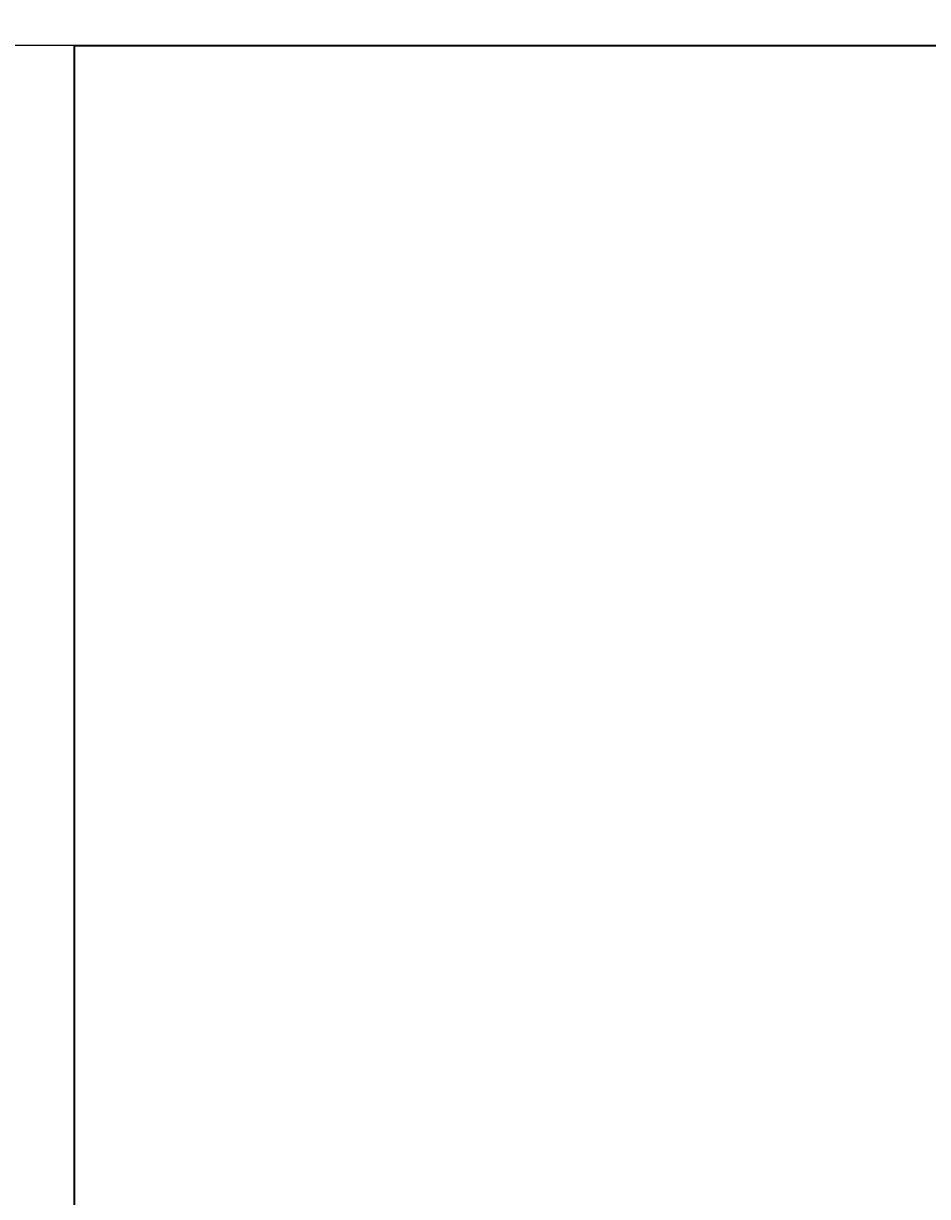
# Model space of a CAD drawing. Units: inches. Extents: x 1770 to 2988, y 1161 to 3221.
# Tile 14 of 44: x 2159 to 2194, y 2323 to 2369. Entities that reach past the tile are written whole.
import ezdxf

# ---------------------------------------------------------------- set-up
doc = ezdxf.new("R2010")
doc.units = ezdxf.units.IN
doc.layers.add('A-ANNO-DIMS', color=2, linetype='Continuous', lineweight=18)
doc.layers.add('A-WALL', color=7, linetype='Continuous', lineweight=35)
doc.styles.get("Standard").update_dxf_attribs({"font": 'arial.ttf'})
doc.dimstyles.get("Standard").update_dxf_attribs({"dimtxt": 0.18, "dimasz": 0.18, "dimexe": 0.18, "dimexo": 0.0625, "dimgap": 0.09, "dimtad": 0, "dimtih": 1, "dimtoh": 1, "dimdec": 4, "dimzin": 0, "dimdsep": 46, "dimtxsty": 'Standard', "dimcen": 0.09, "dimadec": 0, "dimazin": 0, "dimtfac": 1, "dimtdec": 4, "dimtofl": 0, "dimtmove": 0, "dimatfit": 3, "dimfxl": 1, "dimtolj": 1, "dimtzin": 0, "dimarcsym": 0})

# ---------------------------------------------------------------- blocks, each defined once
blk = doc.blocks.new('*D73')
at = {"layer": 'A-ANNO-DIMS', "color": 0, "lineweight": -2, "transparency": 16777216}
for p, q in [((2456.133, 2367.702), (1907.104, 2367.702)), ((1907.284, 2367.522), (1907.284, 2319.884)), ((1907.284, 2271.882), (1907.284, 2319.52)), ((2456.133, 2271.702), (1907.104, 2271.702))]:
    blk.add_line(p, q, dxfattribs=at)
at = {"layer": 'A-ANNO-DIMS', "color": 0, "transparency": 16777216}
for points in [[(1907.254, 2367.522), (1907.314, 2367.522), (1907.284, 2367.702)], [(1907.254, 2271.882), (1907.314, 2271.882), (1907.284, 2271.702)]]:
    blk.add_solid(points, dxfattribs=at)
at = {"layer": 'Defpoints', "color": 0, "transparency": 16777216}
for p in [(1907.284, 2367.702), (2456.196, 2367.702), (2456.196, 2271.702)]:
    blk.add_point(p, dxfattribs=at)
at = {"layer": 'A-ANNO-DIMS', "color": 0, "transparency": 16777216, "insert": (1907.284, 2319.702), "char_height": 0.18, "attachment_point": 5}
blk.add_mtext('\\A1;96', dxfattribs=at)
blk = doc.blocks.new('*D79')
at = {"layer": 'A-ANNO-DIMS', "color": 0, "lineweight": -2, "transparency": 16777216}
for p, q in [((2151.696, 1610.265), (2151.696, 2570.705)), ((2151.876, 2570.525), (2177.783, 2570.525)), ((2204.477, 2570.525), (2178.57, 2570.525)), ((2204.657, 1610.265), (2204.657, 2570.705))]:
    blk.add_line(p, q, dxfattribs=at)
at = {"layer": 'A-ANNO-DIMS', "color": 0, "transparency": 16777216}
for points in [[(2151.876, 2570.555), (2151.876, 2570.495), (2151.696, 2570.525)], [(2204.477, 2570.555), (2204.477, 2570.495), (2204.657, 2570.525)]]:
    blk.add_solid(points, dxfattribs=at)
at = {"layer": 'Defpoints', "color": 0, "transparency": 16777216}
for p in [(2204.657, 2570.525), (2151.696, 1610.202), (2204.657, 1610.202)]:
    blk.add_point(p, dxfattribs=at)
at = {"layer": 'A-ANNO-DIMS', "color": 0, "transparency": 16777216, "insert": (2178.176, 2570.525), "char_height": 0.18, "attachment_point": 5}
blk.add_mtext('\\A1;52.96', dxfattribs=at)

msp = doc.modelspace()

# ---------------------------------------------------------------- linework, layer by layer
at = {"layer": 'A-WALL'}
for q in [(2328.696, 2367.7021), (2160.696, 2175.7021)]:
    msp.add_line((2160.696, 2367.7021), q, dxfattribs=at)

# ---------------------------------------------------------------- dimensions: what is measured, and where the dimension line sits
at = {"layer": 'A-ANNO-DIMS'}
dim = msp.add_linear_dim(base=(2204.6568, 2570.5247), p1=(2151.696, 1610.2021), p2=(2204.6568, 1610.2021), dimstyle='Standard', override={"dimdec": 2, "dimlfac": 1, "dimrnd": 0, "dimzin": 0, "dimdsep": 46, "dimlunit": 2}, dxfattribs=at)
dim.commit()
dim.dimension.update_dxf_attribs({"geometry": '*D79', "text_midpoint": (2178.1764, 2570.5247)})
dim = msp.add_linear_dim(base=(1907.2844, 2367.7021), p1=(2456.196, 2271.7021), p2=(2456.196, 2367.7021), angle=90, dimstyle='Standard', override={"dimdec": 0, "dimlfac": 1, "dimrnd": 0, "dimzin": 0, "dimdsep": 46, "dimlunit": 2}, dxfattribs=at)
dim.commit()
dim.dimension.update_dxf_attribs({"geometry": '*D73', "text_midpoint": (1907.2844, 2319.7021)})

doc.saveas('drawing.dxf')
